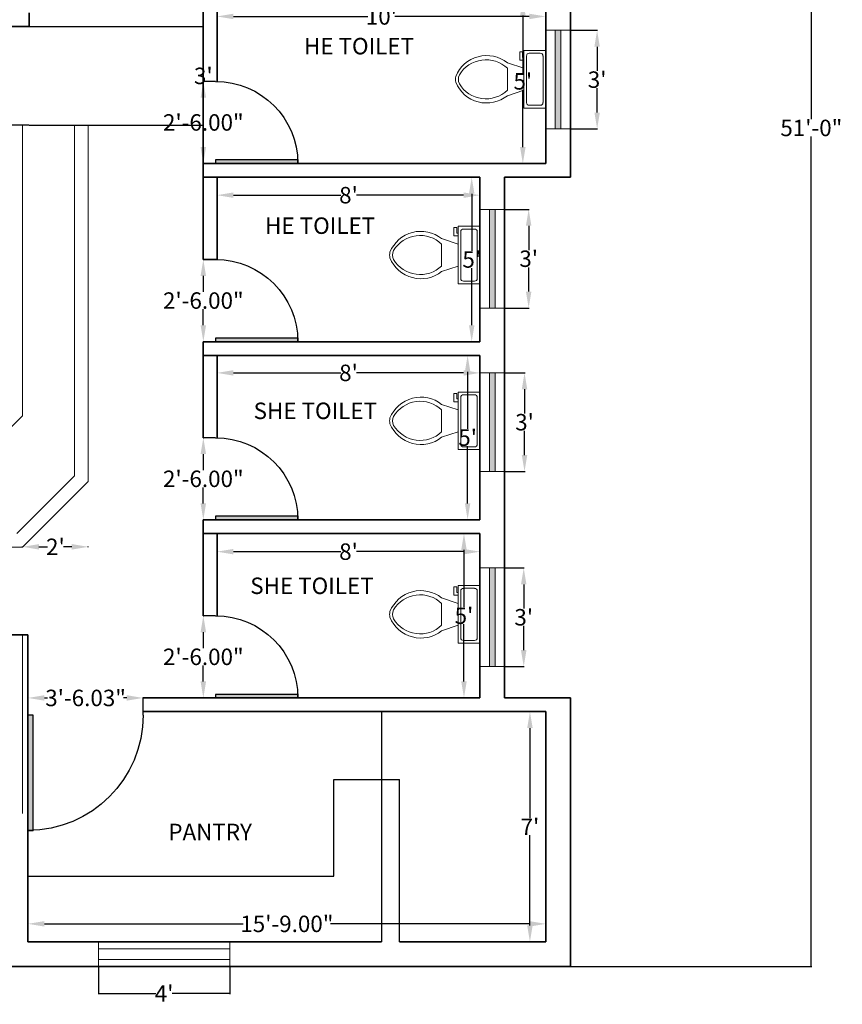
# Model space of a CAD drawing. Units: inches. Extents: x -57 to 1512, y -896 to 149.
# Tile 5 of 6: x 1211 to 1512, y -620 to -261. Entities that reach past the tile are written whole.
import ezdxf

# ---------------------------------------------------------------- set-up
doc = ezdxf.new("R2010")
doc.units = ezdxf.units.IN
doc.header["$MEASUREMENT"] = 0
doc.layers.get('Defpoints').update_dxf_attribs({"color": 9})
for name, color, linetype, lineweight in [('A-ANNO-DIMS', 2, 'Continuous', 18), ('A-AREA-IDEN', 7, 'Continuous', 18), ('A-DOOR', 3, 'Continuous', 25), ('A-DOOR-PATT', 3, 'Continuous', 13), ('A-FLOR-CASE', 8, 'Continuous', 25), ('A-FLOR-FIXT', 9, 'Continuous', 18), ('A-FURN', 8, 'Continuous', 18), ('A-GLAZ', 4, 'Continuous', 18), ('A-GLAZ-PATT', 4, 'Continuous', 13), ('A-WALL', 7, 'Continuous', 35)]:
    doc.layers.add(name, color=color, linetype=linetype, lineweight=lineweight)
doc.styles.get("Standard").update_dxf_attribs({"font": 'arial.ttf'})
doc.dimstyles.get("Standard").update_dxf_attribs({"dimtxt": 6, "dimasz": 0.18, "dimexe": 0.18, "dimexo": 0.0625, "dimgap": 0.09, "dimtad": 0, "dimtih": 1, "dimtoh": 1, "dimzin": 0, "dimdsep": 46, "dimlunit": 3, "dimtxsty": 'Standard', "dimcen": 0.09, "dimadec": 0, "dimazin": 0, "dimtfac": 1, "dimtofl": 0, "dimtmove": 0, "dimatfit": 3, "dimfxl": 1, "dimtolj": 1, "dimtzin": 0, "dimarcsym": 0})

# ---------------------------------------------------------------- blocks, each defined once
blk = doc.blocks.new('*U2')
for p, q in [((0, 0), (0, -6)), ((40, 0), (40, -6))]:
    blk.add_line(p, q)
blk.add_lwpolyline([(0, 0), (0, 40), (1.75, 40), (1.75, 0)], close=True)
blk.add_arc((0, 0), 40, 0, 90)
blk = doc.blocks.new('*D30')
at = {"layer": 'A-ANNO-DIMS', "color": 0, "lineweight": -2, "transparency": 16777216}
for p, q in [((1214.47, -508.36), (1214.47, -508.24)), ((1220.47, -508.42), (1221.6, -508.42)), ((1250.5, -508.42), (1249.37, -508.42)), ((1256.5, -508.36), (1256.5, -508.24))]:
    blk.add_line(p, q, dxfattribs=at)
at = {"layer": 'A-ANNO-DIMS', "color": 0, "transparency": 16777216}
for points in [[(1220.47, -507.42), (1220.47, -509.42), (1214.47, -508.42)], [(1250.5, -507.42), (1250.5, -509.42), (1256.5, -508.42)]]:
    blk.add_solid(points, dxfattribs=at)
at = {"layer": 'Defpoints', "color": 0, "transparency": 16777216}
for p in [(1214.47, -508.42), (1214.47, -508.42), (1256.5, -508.42)]:
    blk.add_point(p, dxfattribs=at)
at = {"layer": 'A-ANNO-DIMS', "color": 0, "transparency": 16777216, "insert": (1235.49, -508.42), "char_height": 6, "attachment_point": 5}
blk.add_mtext('\\A1;3\'-6.03"', dxfattribs=at)
blk = doc.blocks.new('*D31')
at = {"layer": 'A-ANNO-DIMS', "color": 0, "lineweight": -2, "transparency": 16777216}
for p, q in [((1278.53, -478.42), (1278.65, -478.42)), ((1278.47, -484.42), (1278.47, -490.27)), ((1278.47, -502.42), (1278.47, -496.58)), ((1278.53, -508.42), (1278.65, -508.42))]:
    blk.add_line(p, q, dxfattribs=at)
at = {"layer": 'A-ANNO-DIMS', "color": 0, "transparency": 16777216}
for points in [[(1277.47, -484.42), (1279.47, -484.42), (1278.47, -478.42)], [(1277.47, -502.42), (1279.47, -502.42), (1278.47, -508.42)]]:
    blk.add_solid(points, dxfattribs=at)
at = {"layer": 'Defpoints', "color": 0, "transparency": 16777216}
for p in [(1278.47, -478.42), (1278.47, -508.42), (1278.47, -508.42)]:
    blk.add_point(p, dxfattribs=at)
at = {"layer": 'A-ANNO-DIMS', "color": 0, "transparency": 16777216, "insert": (1278.47, -493.42), "char_height": 6, "attachment_point": 5}
blk.add_mtext('\\A1;2\'-6.00"', dxfattribs=at)
blk = doc.blocks.new('*D32')
at = {"layer": 'A-ANNO-DIMS', "color": 0, "lineweight": -2, "transparency": 16777216}
for p, q in [((1278.53, -413.46), (1278.65, -413.46)), ((1278.47, -419.46), (1278.47, -425.31)), ((1278.47, -437.46), (1278.47, -431.61)), ((1278.53, -443.46), (1278.65, -443.46))]:
    blk.add_line(p, q, dxfattribs=at)
at = {"layer": 'A-ANNO-DIMS', "color": 0, "transparency": 16777216}
for points in [[(1277.47, -419.46), (1279.47, -419.46), (1278.47, -413.46)], [(1277.47, -437.46), (1279.47, -437.46), (1278.47, -443.46)]]:
    blk.add_solid(points, dxfattribs=at)
at = {"layer": 'Defpoints', "color": 0, "transparency": 16777216}
for p in [(1278.47, -413.46), (1278.47, -443.46), (1278.47, -443.46)]:
    blk.add_point(p, dxfattribs=at)
at = {"layer": 'A-ANNO-DIMS', "color": 0, "transparency": 16777216, "insert": (1278.47, -428.46), "char_height": 6, "attachment_point": 5}
blk.add_mtext('\\A1;2\'-6.00"', dxfattribs=at)
blk = doc.blocks.new('*D33')
at = {"layer": 'A-ANNO-DIMS', "color": 0, "lineweight": -2, "transparency": 16777216}
for p, q in [((1278.53, -348.42), (1278.65, -348.42)), ((1278.47, -354.42), (1278.47, -360.27)), ((1278.47, -372.42), (1278.47, -366.58)), ((1278.53, -378.42), (1278.65, -378.42))]:
    blk.add_line(p, q, dxfattribs=at)
at = {"layer": 'A-ANNO-DIMS', "color": 0, "transparency": 16777216}
for points in [[(1277.47, -354.42), (1279.47, -354.42), (1278.47, -348.42)], [(1277.47, -372.42), (1279.47, -372.42), (1278.47, -378.42)]]:
    blk.add_solid(points, dxfattribs=at)
at = {"layer": 'Defpoints', "color": 0, "transparency": 16777216}
for p in [(1278.47, -348.42), (1278.47, -378.42), (1278.47, -378.42)]:
    blk.add_point(p, dxfattribs=at)
at = {"layer": 'A-ANNO-DIMS', "color": 0, "transparency": 16777216, "insert": (1278.47, -363.42), "char_height": 6, "attachment_point": 5}
blk.add_mtext('\\A1;2\'-6.00"', dxfattribs=at)
blk = doc.blocks.new('*D34')
at = {"layer": 'A-ANNO-DIMS', "color": 0, "lineweight": -2, "transparency": 16777216}
for p, q in [((1278.53, -283.42), (1278.65, -283.42)), ((1278.47, -289.42), (1278.47, -295.27)), ((1278.47, -307.42), (1278.47, -301.58)), ((1278.53, -313.42), (1278.65, -313.42))]:
    blk.add_line(p, q, dxfattribs=at)
at = {"layer": 'A-ANNO-DIMS', "color": 0, "transparency": 16777216}
for points in [[(1277.47, -289.42), (1279.47, -289.42), (1278.47, -283.42)], [(1277.47, -307.42), (1279.47, -307.42), (1278.47, -313.42)]]:
    blk.add_solid(points, dxfattribs=at)
at = {"layer": 'Defpoints', "color": 0, "transparency": 16777216}
for p in [(1278.47, -283.42), (1278.47, -313.42), (1278.47, -313.42)]:
    blk.add_point(p, dxfattribs=at)
at = {"layer": 'A-ANNO-DIMS', "color": 0, "transparency": 16777216, "insert": (1278.47, -298.42), "char_height": 6, "attachment_point": 5}
blk.add_mtext('\\A1;2\'-6.00"', dxfattribs=at)
blk = doc.blocks.new('*D44')
at = {"layer": 'A-ANNO-DIMS', "color": 0, "lineweight": -2, "transparency": 16777216}
for p, q in [((1240.15, -606.48), (1240.15, -616.46)), ((1288.15, -606.48), (1288.15, -616.46)), ((1240.33, -616.28), (1261.17, -616.28)), ((1287.97, -616.28), (1267.12, -616.28))]:
    blk.add_line(p, q, dxfattribs=at)
at = {"layer": 'A-ANNO-DIMS', "color": 0, "transparency": 16777216}
for points in [[(1240.33, -616.25), (1240.33, -616.31), (1240.15, -616.28)], [(1287.97, -616.25), (1287.97, -616.31), (1288.15, -616.28)]]:
    blk.add_solid(points, dxfattribs=at)
at = {"layer": 'Defpoints', "color": 0, "transparency": 16777216}
for p in [(1240.15, -606.42), (1288.15, -606.42), (1288.15, -616.28)]:
    blk.add_point(p, dxfattribs=at)
at = {"layer": 'A-ANNO-DIMS', "color": 0, "transparency": 16777216, "insert": (1264.15, -616.28), "char_height": 6, "attachment_point": 5}
blk.add_mtext("\\A1;4'", dxfattribs=at)
blk = doc.blocks.new('*D45')
at = {"layer": 'A-ANNO-DIMS', "color": 0, "lineweight": -2, "transparency": 16777216}
for p, q in [((1388.53, -330.14), (1397.42, -330.14)), ((1397.24, -336.14), (1397.24, -344.99)), ((1397.24, -360.14), (1397.24, -351.3)), ((1388.53, -366.14), (1397.42, -366.14))]:
    blk.add_line(p, q, dxfattribs=at)
at = {"layer": 'A-ANNO-DIMS', "color": 0, "transparency": 16777216}
for points in [[(1396.24, -336.14), (1398.24, -336.14), (1397.24, -330.14)], [(1396.24, -360.14), (1398.24, -360.14), (1397.24, -366.14)]]:
    blk.add_solid(points, dxfattribs=at)
at = {"layer": 'Defpoints', "color": 0, "transparency": 16777216}
for p in [(1388.47, -330.14), (1388.47, -366.14), (1397.24, -366.14)]:
    blk.add_point(p, dxfattribs=at)
at = {"layer": 'A-ANNO-DIMS', "color": 0, "transparency": 16777216, "insert": (1397.24, -348.14), "char_height": 6, "attachment_point": 5}
blk.add_mtext("\\A1;3'", dxfattribs=at)
blk = doc.blocks.new('*D46')
at = {"layer": 'A-ANNO-DIMS', "color": 0, "lineweight": -2, "transparency": 16777216}
for p, q in [((1388.53, -389.8), (1395.91, -389.8)), ((1395.73, -395.8), (1395.73, -404.65)), ((1395.73, -419.8), (1395.73, -410.96)), ((1388.53, -425.8), (1395.91, -425.8))]:
    blk.add_line(p, q, dxfattribs=at)
at = {"layer": 'A-ANNO-DIMS', "color": 0, "transparency": 16777216}
for points in [[(1394.73, -395.8), (1396.73, -395.8), (1395.73, -389.8)], [(1394.73, -419.8), (1396.73, -419.8), (1395.73, -425.8)]]:
    blk.add_solid(points, dxfattribs=at)
at = {"layer": 'Defpoints', "color": 0, "transparency": 16777216}
for p in [(1388.47, -389.8), (1388.47, -425.8), (1395.73, -425.8)]:
    blk.add_point(p, dxfattribs=at)
at = {"layer": 'A-ANNO-DIMS', "color": 0, "transparency": 16777216, "insert": (1395.73, -407.8), "char_height": 6, "attachment_point": 5}
blk.add_mtext("\\A1;3'", dxfattribs=at)
blk = doc.blocks.new('*D47')
at = {"layer": 'A-ANNO-DIMS', "color": 0, "lineweight": -2, "transparency": 16777216}
for p, q in [((1388.53, -460.98), (1395.61, -460.98)), ((1395.43, -466.98), (1395.43, -475.83)), ((1395.43, -490.98), (1395.43, -482.14)), ((1388.53, -496.98), (1395.61, -496.98))]:
    blk.add_line(p, q, dxfattribs=at)
at = {"layer": 'A-ANNO-DIMS', "color": 0, "transparency": 16777216}
for points in [[(1394.43, -466.98), (1396.43, -466.98), (1395.43, -460.98)], [(1394.43, -490.98), (1396.43, -490.98), (1395.43, -496.98)]]:
    blk.add_solid(points, dxfattribs=at)
at = {"layer": 'Defpoints', "color": 0, "transparency": 16777216}
for p in [(1388.47, -460.98), (1395.43, -460.98), (1388.47, -496.98)]:
    blk.add_point(p, dxfattribs=at)
at = {"layer": 'A-ANNO-DIMS', "color": 0, "transparency": 16777216, "insert": (1395.43, -478.98), "char_height": 6, "attachment_point": 5}
blk.add_mtext("\\A1;3'", dxfattribs=at)
blk = doc.blocks.new('*D48')
at = {"layer": 'A-ANNO-DIMS', "color": 0, "lineweight": -2, "transparency": 16777216}
for p, q in [((1412.53, -264.79), (1422.41, -264.79)), ((1422.23, -270.79), (1422.23, -279.64)), ((1422.23, -294.79), (1422.23, -285.95)), ((1412.53, -300.79), (1422.41, -300.79))]:
    blk.add_line(p, q, dxfattribs=at)
at = {"layer": 'A-ANNO-DIMS', "color": 0, "transparency": 16777216}
for points in [[(1421.23, -270.79), (1423.23, -270.79), (1422.23, -264.79)], [(1421.23, -294.79), (1423.23, -294.79), (1422.23, -300.79)]]:
    blk.add_solid(points, dxfattribs=at)
at = {"layer": 'Defpoints', "color": 0, "transparency": 16777216}
for p in [(1412.47, -264.79), (1412.47, -300.79), (1422.23, -300.79)]:
    blk.add_point(p, dxfattribs=at)
at = {"layer": 'A-ANNO-DIMS', "color": 0, "transparency": 16777216, "insert": (1422.23, -282.79), "char_height": 6, "attachment_point": 5}
blk.add_mtext("\\A1;3'", dxfattribs=at)
blk = doc.blocks.new('*U24')
for p, q in [((9.5, -6), (9.5, -2)), ((-10, -8.5), (-8, -8.5)), ((-10, -9.5), (-10, -8.5)), ((-7, -9.5), (-10, -9.5)), ((-8, -8.5), (-8, -8)), ((-7, -8), (-7, -9.5)), ((-4, -8), (-6, -14)), ((4, -8), (6, -14)), ((4, -14), (-4, -14))]:
    blk.add_line(p, q)
blk.add_lwpolyline([(10.5, -8), (10.5, 0), (-10.5, 0), (-10.5, -8)], close=True)
for points in [[(-9.5, -2), (-9.5, -6)], [(8.5, -1), (-8.5, -1)], [(-8.5, -7), (8.5, -7)]]:
    blk.add_lwpolyline(points)
for centre, radius, start, end in [((-8.62, -1.88), 0.884, 81.8699, 188.1301), ((8.62, -1.88), 0.884, 351.8699, 98.1301), ((-8.62, -6.12), 0.884, 171.8699, 278.1301), ((8.62, -6.12), 0.884, 261.8699, 8.1301), ((3.52, -21.58), 12.17, 141.4691, 247.9714), ((4.2, -21.82), 11.33, 136.3677, 238.9468), ((-3.52, -21.58), 12.17, 292.0284, 38.5307), ((-4.2, -21.82), 11.33, 301.053, 43.6321), ((0, -27.88), 4, 245.7318, 294.2682), ((0, -29), 4, 254.8605, 285.1395)]:
    blk.add_arc(centre, radius, start, end)
blk = doc.blocks.new('*D57')
at = {"layer": 'A-ANNO-DIMS', "color": 0, "lineweight": -2, "transparency": 16777216}
for p, q in [((1214.95, -263.42), (1278.65, -263.42)), ((1278.47, -263.6), (1278.47, -278.27)), ((1278.47, -299.24), (1278.47, -284.58)), ((1214.95, -299.42), (1278.65, -299.42))]:
    blk.add_line(p, q, dxfattribs=at)
at = {"layer": 'A-ANNO-DIMS', "color": 0, "transparency": 16777216}
for points in [[(1278.44, -263.6), (1278.5, -263.6), (1278.47, -263.42)], [(1278.44, -299.24), (1278.5, -299.24), (1278.47, -299.42)]]:
    blk.add_solid(points, dxfattribs=at)
at = {"layer": 'Defpoints', "color": 0, "transparency": 16777216}
for p in [(1214.89, -263.42), (1214.89, -299.42), (1278.47, -299.42)]:
    blk.add_point(p, dxfattribs=at)
at = {"layer": 'A-ANNO-DIMS', "color": 0, "transparency": 16777216, "insert": (1278.47, -281.42), "char_height": 6, "attachment_point": 5}
blk.add_mtext("\\A1;3'", dxfattribs=at)
blk = doc.blocks.new('*D58')
at = {"layer": 'A-ANNO-DIMS', "color": 0, "lineweight": -2, "transparency": 16777216}
for p, q in [((1214.83, -263.42), (1191.49, -263.42)), ((1191.67, -269.42), (1191.67, -278.27)), ((1191.67, -293.42), (1191.67, -284.58)), ((1214.83, -299.42), (1191.49, -299.42))]:
    blk.add_line(p, q, dxfattribs=at)
at = {"layer": 'A-ANNO-DIMS', "color": 0, "transparency": 16777216}
for points in [[(1190.67, -269.42), (1192.67, -269.42), (1191.67, -263.42)], [(1190.67, -293.42), (1192.67, -293.42), (1191.67, -299.42)]]:
    blk.add_solid(points, dxfattribs=at)
at = {"layer": 'Defpoints', "color": 0, "transparency": 16777216}
for p in [(1214.89, -263.42), (1191.67, -299.42), (1214.89, -299.42)]:
    blk.add_point(p, dxfattribs=at)
at = {"layer": 'A-ANNO-DIMS', "color": 0, "transparency": 16777216, "insert": (1191.67, -281.42), "char_height": 6, "attachment_point": 5}
blk.add_mtext("\\A1;3'", dxfattribs=at)
blk = doc.blocks.new('*D61')
at = {"layer": 'A-ANNO-DIMS', "color": 0, "lineweight": -2, "transparency": 16777216}
for p, q in [((1212.47, -453.36), (1212.47, -453.1)), ((1218.47, -453.28), (1221.57, -453.28)), ((1230.47, -453.28), (1227.37, -453.28)), ((1236.47, -453.36), (1236.47, -453.1))]:
    blk.add_line(p, q, dxfattribs=at)
at = {"layer": 'A-ANNO-DIMS', "color": 0, "transparency": 16777216}
for points in [[(1218.47, -452.28), (1218.47, -454.28), (1212.47, -453.28)], [(1230.47, -452.28), (1230.47, -454.28), (1236.47, -453.28)]]:
    blk.add_solid(points, dxfattribs=at)
at = {"layer": 'Defpoints', "color": 0, "transparency": 16777216}
for p in [(1212.47, -453.42), (1236.47, -453.28), (1236.47, -453.42)]:
    blk.add_point(p, dxfattribs=at)
at = {"layer": 'A-ANNO-DIMS', "color": 0, "transparency": 16777216, "insert": (1224.47, -453.28), "char_height": 6, "attachment_point": 5}
blk.add_mtext("\\A1;2'", dxfattribs=at)
blk = doc.blocks.new('*D62')
at = {"layer": 'A-ANNO-DIMS', "color": 0, "lineweight": -2, "transparency": 16777216}
for p, q in [((1283.47, -253.48), (1283.47, -259.92)), ((1403.47, -253.48), (1403.47, -259.92)), ((1289.47, -259.74), (1338.57, -259.74)), ((1397.47, -259.74), (1348.37, -259.74))]:
    blk.add_line(p, q, dxfattribs=at)
at = {"layer": 'A-ANNO-DIMS', "color": 0, "transparency": 16777216}
for points in [[(1289.47, -258.74), (1289.47, -260.74), (1283.47, -259.74)], [(1397.47, -258.74), (1397.47, -260.74), (1403.47, -259.74)]]:
    blk.add_solid(points, dxfattribs=at)
at = {"layer": 'Defpoints', "color": 0, "transparency": 16777216}
for p in [(1283.47, -253.42), (1403.47, -253.42), (1403.47, -259.74)]:
    blk.add_point(p, dxfattribs=at)
at = {"layer": 'A-ANNO-DIMS', "color": 0, "transparency": 16777216, "insert": (1343.47, -259.74), "char_height": 6, "attachment_point": 5}
blk.add_mtext("\\A1;10'", dxfattribs=at)
blk = doc.blocks.new('*D63')
at = {"layer": 'A-ANNO-DIMS', "color": 0, "lineweight": -2, "transparency": 16777216}
for p, q in [((1403.41, -253.42), (1394.93, -253.42)), ((1395.11, -259.42), (1395.11, -280.28)), ((1395.11, -307.42), (1395.11, -286.56)), ((1403.41, -313.42), (1394.93, -313.42))]:
    blk.add_line(p, q, dxfattribs=at)
at = {"layer": 'A-ANNO-DIMS', "color": 0, "transparency": 16777216}
for points in [[(1394.11, -259.42), (1396.11, -259.42), (1395.11, -253.42)], [(1394.11, -307.42), (1396.11, -307.42), (1395.11, -313.42)]]:
    blk.add_solid(points, dxfattribs=at)
at = {"layer": 'Defpoints', "color": 0, "transparency": 16777216}
for p in [(1395.11, -253.42), (1403.47, -253.42), (1403.47, -313.42)]:
    blk.add_point(p, dxfattribs=at)
at = {"layer": 'A-ANNO-DIMS', "color": 0, "transparency": 16777216, "insert": (1395.11, -283.42), "char_height": 6, "attachment_point": 5}
blk.add_mtext("\\A1;5'", dxfattribs=at)
blk = doc.blocks.new('*D64')
at = {"layer": 'A-ANNO-DIMS', "color": 0, "lineweight": -2, "transparency": 16777216}
for p, q in [((1283.47, -324.89), (1283.47, -324.77)), ((1289.47, -324.95), (1328.62, -324.95)), ((1373.47, -324.95), (1334.33, -324.95)), ((1379.47, -324.89), (1379.47, -324.77))]:
    blk.add_line(p, q, dxfattribs=at)
at = {"layer": 'A-ANNO-DIMS', "color": 0, "transparency": 16777216}
for points in [[(1289.47, -323.95), (1289.47, -325.95), (1283.47, -324.95)], [(1373.47, -323.95), (1373.47, -325.95), (1379.47, -324.95)]]:
    blk.add_solid(points, dxfattribs=at)
at = {"layer": 'Defpoints', "color": 0, "transparency": 16777216}
for p in [(1283.47, -324.95), (1379.47, -324.95), (1379.47, -324.95)]:
    blk.add_point(p, dxfattribs=at)
at = {"layer": 'A-ANNO-DIMS', "color": 0, "transparency": 16777216, "insert": (1331.47, -324.95), "char_height": 6, "attachment_point": 5}
blk.add_mtext("\\A1;8'", dxfattribs=at)
blk = doc.blocks.new('*D65')
at = {"layer": 'A-ANNO-DIMS', "color": 0, "lineweight": -2, "transparency": 16777216}
for p, q in [((1379.41, -318.42), (1376.27, -318.42)), ((1376.45, -324.42), (1376.45, -345.28)), ((1376.45, -372.42), (1376.45, -351.56)), ((1379.41, -378.42), (1376.27, -378.42))]:
    blk.add_line(p, q, dxfattribs=at)
at = {"layer": 'A-ANNO-DIMS', "color": 0, "transparency": 16777216}
for points in [[(1375.45, -324.42), (1377.45, -324.42), (1376.45, -318.42)], [(1375.45, -372.42), (1377.45, -372.42), (1376.45, -378.42)]]:
    blk.add_solid(points, dxfattribs=at)
at = {"layer": 'Defpoints', "color": 0, "transparency": 16777216}
for p in [(1379.47, -318.42), (1376.45, -378.42), (1379.47, -378.42)]:
    blk.add_point(p, dxfattribs=at)
at = {"layer": 'A-ANNO-DIMS', "color": 0, "transparency": 16777216, "insert": (1376.45, -348.42), "char_height": 6, "attachment_point": 5}
blk.add_mtext("\\A1;5'", dxfattribs=at)
blk = doc.blocks.new('*D66')
at = {"layer": 'A-ANNO-DIMS', "color": 0, "lineweight": -2, "transparency": 16777216}
for p, q in [((1379.41, -383.42), (1374.77, -383.42)), ((1374.95, -389.42), (1374.95, -410.28)), ((1374.95, -437.42), (1374.95, -416.56)), ((1379.41, -443.42), (1374.77, -443.42))]:
    blk.add_line(p, q, dxfattribs=at)
at = {"layer": 'A-ANNO-DIMS', "color": 0, "transparency": 16777216}
for points in [[(1373.95, -389.42), (1375.95, -389.42), (1374.95, -383.42)], [(1373.95, -437.42), (1375.95, -437.42), (1374.95, -443.42)]]:
    blk.add_solid(points, dxfattribs=at)
at = {"layer": 'Defpoints', "color": 0, "transparency": 16777216}
for p in [(1379.47, -383.42), (1374.95, -443.42), (1379.47, -443.42)]:
    blk.add_point(p, dxfattribs=at)
at = {"layer": 'A-ANNO-DIMS', "color": 0, "transparency": 16777216, "insert": (1374.95, -413.42), "char_height": 6, "attachment_point": 5}
blk.add_mtext("\\A1;5'", dxfattribs=at)
blk = doc.blocks.new('*D67')
at = {"layer": 'A-ANNO-DIMS', "color": 0, "lineweight": -2, "transparency": 16777216}
for p, q in [((1379.41, -448.42), (1373.44, -448.42)), ((1373.62, -454.42), (1373.62, -475.28)), ((1373.62, -502.42), (1373.62, -481.56)), ((1379.41, -508.42), (1373.44, -508.42))]:
    blk.add_line(p, q, dxfattribs=at)
at = {"layer": 'A-ANNO-DIMS', "color": 0, "transparency": 16777216}
for points in [[(1372.62, -454.42), (1374.62, -454.42), (1373.62, -448.42)], [(1372.62, -502.42), (1374.62, -502.42), (1373.62, -508.42)]]:
    blk.add_solid(points, dxfattribs=at)
at = {"layer": 'Defpoints', "color": 0, "transparency": 16777216}
for p in [(1379.47, -448.42), (1373.62, -508.42), (1379.47, -508.42)]:
    blk.add_point(p, dxfattribs=at)
at = {"layer": 'A-ANNO-DIMS', "color": 0, "transparency": 16777216, "insert": (1373.62, -478.42), "char_height": 6, "attachment_point": 5}
blk.add_mtext("\\A1;5'", dxfattribs=at)
blk = doc.blocks.new('*D68')
at = {"layer": 'A-ANNO-DIMS', "color": 0, "lineweight": -2, "transparency": 16777216}
for p, q in [((1283.47, -383.48), (1283.47, -389.98)), ((1379.47, -383.66), (1379.47, -389.98)), ((1289.47, -389.8), (1328.62, -389.8)), ((1373.47, -389.8), (1334.33, -389.8))]:
    blk.add_line(p, q, dxfattribs=at)
at = {"layer": 'A-ANNO-DIMS', "color": 0, "transparency": 16777216}
for points in [[(1289.47, -388.8), (1289.47, -390.8), (1283.47, -389.8)], [(1373.47, -388.8), (1373.47, -390.8), (1379.47, -389.8)]]:
    blk.add_solid(points, dxfattribs=at)
at = {"layer": 'Defpoints', "color": 0, "transparency": 16777216}
for p in [(1283.47, -383.42), (1379.47, -383.6), (1379.47, -389.8)]:
    blk.add_point(p, dxfattribs=at)
at = {"layer": 'A-ANNO-DIMS', "color": 0, "transparency": 16777216, "insert": (1331.47, -389.8), "char_height": 6, "attachment_point": 5}
blk.add_mtext("\\A1;8'", dxfattribs=at)
blk = doc.blocks.new('*D69')
at = {"layer": 'A-ANNO-DIMS', "color": 0, "lineweight": -2, "transparency": 16777216}
for p, q in [((1283.47, -448.48), (1283.47, -455.22)), ((1379.47, -448.48), (1379.47, -455.22)), ((1289.47, -455.04), (1328.62, -455.04)), ((1373.47, -455.04), (1334.33, -455.04))]:
    blk.add_line(p, q, dxfattribs=at)
at = {"layer": 'A-ANNO-DIMS', "color": 0, "transparency": 16777216}
for points in [[(1289.47, -454.04), (1289.47, -456.04), (1283.47, -455.04)], [(1373.47, -454.04), (1373.47, -456.04), (1379.47, -455.04)]]:
    blk.add_solid(points, dxfattribs=at)
at = {"layer": 'Defpoints', "color": 0, "transparency": 16777216}
for p in [(1283.47, -448.42), (1379.47, -448.42), (1379.47, -455.04)]:
    blk.add_point(p, dxfattribs=at)
at = {"layer": 'A-ANNO-DIMS', "color": 0, "transparency": 16777216, "insert": (1331.47, -455.04), "char_height": 6, "attachment_point": 5}
blk.add_mtext("\\A1;8'", dxfattribs=at)
blk = doc.blocks.new('*D70')
at = {"layer": 'A-ANNO-DIMS', "color": 0, "lineweight": -2, "transparency": 16777216}
for p, q in [((1214.47, -597.36), (1214.47, -590.68)), ((1220.47, -590.86), (1293.03, -590.86)), ((1397.47, -590.86), (1324.91, -590.86)), ((1403.47, -597.36), (1403.47, -590.68))]:
    blk.add_line(p, q, dxfattribs=at)
at = {"layer": 'A-ANNO-DIMS', "color": 0, "transparency": 16777216}
for points in [[(1220.47, -589.86), (1220.47, -591.86), (1214.47, -590.86)], [(1397.47, -589.86), (1397.47, -591.86), (1403.47, -590.86)]]:
    blk.add_solid(points, dxfattribs=at)
at = {"layer": 'Defpoints', "color": 0, "transparency": 16777216}
for p in [(1403.47, -590.86), (1214.47, -597.42), (1403.47, -597.42)]:
    blk.add_point(p, dxfattribs=at)
at = {"layer": 'A-ANNO-DIMS', "color": 0, "transparency": 16777216, "insert": (1308.97, -590.86), "char_height": 6, "attachment_point": 5}
blk.add_mtext('\\A1;15\'-9.00"', dxfattribs=at)
blk = doc.blocks.new('*D71')
at = {"layer": 'A-ANNO-DIMS', "color": 0, "lineweight": -2, "transparency": 16777216}
for p, q in [((1403.41, -513.42), (1397.52, -513.42)), ((1397.7, -519.42), (1397.7, -552.33)), ((1397.7, -591.42), (1397.7, -558.51)), ((1403.41, -597.42), (1397.52, -597.42))]:
    blk.add_line(p, q, dxfattribs=at)
at = {"layer": 'A-ANNO-DIMS', "color": 0, "transparency": 16777216}
for points in [[(1396.7, -519.42), (1398.7, -519.42), (1397.7, -513.42)], [(1396.7, -591.42), (1398.7, -591.42), (1397.7, -597.42)]]:
    blk.add_solid(points, dxfattribs=at)
at = {"layer": 'Defpoints', "color": 0, "transparency": 16777216}
for p in [(1397.7, -513.42), (1403.47, -513.42), (1403.47, -597.42)]:
    blk.add_point(p, dxfattribs=at)
at = {"layer": 'A-ANNO-DIMS', "color": 0, "transparency": 16777216, "insert": (1397.7, -555.42), "char_height": 6, "attachment_point": 5}
blk.add_mtext("\\A1;7'", dxfattribs=at)
blk = doc.blocks.new('*D105')
at = {"layer": 'A-ANNO-DIMS', "color": 0, "lineweight": -2, "transparency": 16777216}
for p, q in [((1412.53, 5.58), (1500.6, 5.58)), ((1500.42, 5.4), (1500.42, -297.27)), ((1500.42, -606.24), (1500.42, -303.57)), ((1412.53, -606.42), (1500.6, -606.42))]:
    blk.add_line(p, q, dxfattribs=at)
at = {"layer": 'A-ANNO-DIMS', "color": 0, "transparency": 16777216}
for points in [[(1500.39, 5.4), (1500.45, 5.4), (1500.42, 5.58)], [(1500.39, -606.24), (1500.45, -606.24), (1500.42, -606.42)]]:
    blk.add_solid(points, dxfattribs=at)
at = {"layer": 'Defpoints', "color": 0, "transparency": 16777216}
for p in [(1412.47, 5.58), (1500.42, 5.58), (1412.47, -606.42)]:
    blk.add_point(p, dxfattribs=at)
at = {"layer": 'A-ANNO-DIMS', "color": 0, "transparency": 16777216, "insert": (1500.42, -300.42), "char_height": 6, "attachment_point": 5}
blk.add_mtext('\\A1;51\'-0"', dxfattribs=at)

msp = doc.modelspace()

# ---------------------------------------------------------------- hatches: boundary and pattern name
at = {"layer": 'A-DOOR-PATT'}
h = msp.add_hatch(color=256, dxfattribs=at)
h.dxf.hatch_style = 1
h.paths.add_polyline_path([(1084.811, -453.421), (1053.741, -453.421, 0.0109414), (1053.771, -454.781), (1084.811, -454.781)])
h.paths.add_polyline_path([(1091.31, -491.725), (1089.471, -491.725), (1089.471, -533.753), (1091.31, -533.753)])
h.paths.add_polyline_path([(1216.31, -514.725), (1214.471, -514.725), (1214.471, -556.753, 0.0109414), (1216.31, -556.713)])
h.paths.add_polyline_path([(1312.941, -507.109), (1282.971, -507.109), (1282.971, -508.421), (1312.969, -508.421, 0.0109414)])
h.paths.add_polyline_path([(1312.941, -442.147), (1282.971, -442.147), (1282.971, -443.421), (1312.969, -443.421, 0.0106229)])
h.paths.add_polyline_path([(1302.763, -246.583), (1260.775, -246.583), (1260.775, -248.421), (1302.803, -248.421, 0.0109414)])
h.paths.add_polyline_path([(1312.941, -312.109), (1282.971, -312.109), (1282.971, -313.421), (1312.969, -313.421, 0.0109414)])
h.paths.add_polyline_path([(1312.941, -377.109), (1282.971, -377.109), (1282.971, -378.421), (1312.969, -378.421, 0.0109414)])
h.paths.add_polyline_path([(1061.471, -387.473), (1060.289, -387.473), (1060.289, -414.461, 0.0109414), (1061.471, -414.487)])
h.paths.add_polyline_path([(1060.167, -263.421), (1018.139, -263.421, 0.0109414), (1018.179, -265.26), (1060.167, -265.26)])
h.paths.add_polyline_path([(1326.803, -121.583), (1284.775, -121.583), (1284.775, -123.421), (1326.803, -123.421)])
h.paths.add_polyline_path([(980.763, -121.583), (938.775, -121.583), (938.775, -123.421), (980.803, -123.421, 0.0109414)])
h.paths.add_polyline_path([(1177.375, -188.23), (1115.807, -188.23), (1115.807, -219.221), (1177.375, -219.221)])
at = {"layer": 'A-GLAZ-PATT'}
h = msp.add_hatch(color=256, dxfattribs=at)
h.dxf.hatch_style = 1
h.paths.add_polyline_path([(1408.971, -264.791), (1406.971, -264.791), (1406.971, -300.791), (1408.971, -300.791)])
h.paths.add_polyline_path([(1384.971, -330.143), (1382.971, -330.143), (1382.971, -366.143), (1384.971, -366.143)])
h.paths.add_polyline_path([(1384.971, -460.981), (1382.971, -460.981), (1382.971, -496.981), (1384.971, -496.981)])
h.paths.add_polyline_path([(1384.971, -389.802), (1382.971, -389.802), (1382.971, -425.802), (1384.971, -425.802)])
h.paths.add_polyline_path([(937.971, -469.144), (935.971, -469.144), (935.971, -565.144), (937.971, -565.144)])
h.paths.add_polyline_path([(937.971, -399.584), (935.971, -399.584), (935.971, -435.584), (937.971, -435.584)])

# ---------------------------------------------------------------- linework, layer by layer
at = {"layer": 'A-FLOR-CASE'}
for p, q in [((1343.471, -513.421), (1343.471, -597.421)), ((1326.062, -573.421), (1326.062, -538.172)), ((1326.062, -538.172), (1350.062, -538.172)), ((1350.062, -597.421), (1350.062, -538.172)), ((1214.471, -573.421), (1326.062, -573.421))]:
    msp.add_line(p, q, dxfattribs=at)
at = {"layer": 'A-FURN'}
for p, q in [((1038.48, -299.421), (1278.471, -299.421)), ((1212.471, -405.421), (1212.471, -299.421)), ((1231.471, -299.421), (1231.471, -427.35)), ((1236.471, -299.421), (1236.471, -429.421)), ((1188.471, -429.421), (1212.471, -405.421)), ((1210.4, -448.421), (1231.471, -427.35)), ((1212.471, -453.421), (1236.471, -429.421)), ((1132.471, -453.421), (1212.471, -453.421)), ((1212.471, -485.421), (1212.471, -550.535))]:
    msp.add_line(p, q, dxfattribs=at)
at = {"layer": 'A-GLAZ'}
for p, q in [((1403.471, -264.791), (1412.471, -264.791)), ((1406.971, -264.791), (1406.971, -300.791)), ((1408.971, -264.791), (1408.971, -300.791)), ((1403.471, -300.791), (1412.471, -300.791)), ((1379.471, -330.143), (1388.471, -330.143)), ((1382.971, -330.143), (1382.971, -366.143)), ((1384.971, -330.143), (1384.971, -366.143)), ((1379.471, -366.143), (1388.471, -366.143)), ((1379.471, -389.802), (1388.471, -389.802)), ((1382.971, -389.802), (1382.971, -425.802)), ((1384.971, -389.802), (1384.971, -425.802)), ((1379.471, -425.802), (1388.471, -425.802)), ((1379.471, -460.981), (1388.471, -460.981)), ((1382.971, -460.981), (1382.971, -496.981)), ((1384.971, -460.981), (1384.971, -496.981)), ((1379.471, -496.981), (1388.471, -496.981)), ((1240.146, -597.421), (1240.146, -606.421)), ((1240.146, -599.921), (1288.146, -599.921)), ((1288.146, -597.421), (1288.146, -606.421)), ((1240.146, -603.921), (1288.146, -603.921))]:
    msp.add_line(p, q, dxfattribs=at)
at = {"layer": 'A-WALL'}
for p, q in [((1412.471, 5.579), (1412.471, -318.421)), ((1278.471, -253.421), (1278.471, -348.423)), ((1283.471, -253.421), (1283.471, -283.607)), ((1403.471, -253.421), (1403.471, -313.421)), ((1214.89, -258.421), (1214.89, -263.421)), ((941.471, -263.421), (1214.89, -263.421)), ((1278.471, -313.421), (1403.471, -313.421)), ((1278.471, -318.421), (1379.471, -318.421)), ((1283.471, -318.421), (1283.471, -348.427)), ((1379.471, -318.421), (1379.471, -378.421)), ((1388.471, -318.421), (1388.471, -508.421)), ((1388.471, -318.421), (1412.471, -318.421)), ((1278.475, -348.401), (1283.471, -348.401)), ((1379.471, -348.401), (1379.475, -348.401)), ((1278.471, -378.421), (1379.471, -378.421)), ((1278.471, -378.421), (1278.471, -383.421)), ((1278.471, -383.421), (1379.471, -383.421)), ((1278.471, -383.421), (1278.471, -413.461)), ((1283.471, -383.421), (1283.471, -413.465)), ((1379.471, -383.421), (1379.471, -443.421)), ((1278.471, -443.421), (1379.471, -443.421)), ((1278.471, -443.421), (1278.471, -448.421)), ((1278.471, -448.421), (1379.471, -448.421)), ((1278.471, -448.421), (1278.471, -478.423)), ((1283.471, -448.421), (1283.471, -478.427)), ((1379.471, -448.421), (1379.471, -508.421)), ((1131.471, -485.421), (1214.471, -485.421)), ((1214.471, -485.421), (1214.471, -597.421)), ((1256.499, -508.421), (1379.471, -508.421)), ((1388.471, -508.421), (1412.471, -508.421)), ((1412.471, -508.421), (1412.471, -606.421)), ((1256.499, -513.421), (1403.471, -513.421)), ((1403.471, -513.421), (1403.471, -597.421)), ((1214.471, -597.421), (1343.471, -597.421)), ((1350.062, -597.421), (1403.471, -597.421)), ((932.471, -606.421), (1412.471, -606.421))]:
    msp.add_line(p, q, dxfattribs=at)

# ---------------------------------------------------------------- block references
at = {"layer": 'A-DOOR'}
for p, xscale, yscale, zscale, rotation in [((1282.971, -313.421), -0.7499590753743955, 0.7499590753743955, 0.7499590753743955, 270), ((1282.971, -378.421), -0.7499590753743955, 0.7499590753743955, 0.7499590753743955, 270), ((1282.971, -443.459), -0.7499590753743955, 0.7499590753743955, 0.7499590753743955, 270), ((1282.971, -508.421), -0.7499590753743955, 0.7499590753743955, 0.7499590753743955, 270), ((1214.471, -514.725), -1.050697738247698, 1.050697738247698, 1.050697738247698, 180)]:
    msp.add_blockref('*U2', p, dxfattribs=dict(at, xscale=xscale, yscale=yscale, zscale=zscale, rotation=rotation))
at = {"layer": 'A-FLOR-FIXT', "rotation": 270}
for p in [(1403.471, -282.67), (1379.471, -346.804), (1379.471, -407.308), (1379.471, -477.921)]:
    msp.add_blockref('*U24', p, dxfattribs=at)

# ---------------------------------------------------------------- texts
at = {"layer": 'A-AREA-IDEN', "char_height": 6, "attachment_point": 1}
for s, insert in [('HE TOILET', (1315.209, -267.571)), ('HE TOILET', (1301.039, -333.084)), ('SHE TOILET', (1296.832, -400.65)), ('SHE TOILET', (1295.595, -464.5)), ('PANTRY', (1265.709, -554.323))]:
    msp.add_mtext_dynamic_manual_height_columns(s, width=160.11736, gutter_width=1, heights=[0], dxfattribs=dict(at, insert=insert))

# ---------------------------------------------------------------- dimensions: what is measured, and where the dimension line sits
at = {"layer": 'A-ANNO-DIMS'}
for base, p1, p2, override, picture, middle in [((1500.421, 5.579), (1412.471, -606.421), (1412.471, 5.579), {"dimdec": 1, "dimlfac": 1, "dimrnd": 0, "dimzin": 1, "dimdsep": 46, "dimlunit": 4, "dimfrac": 2}, '*D105', (1500.421, -300.421)), ((1395.11, -253.421), (1403.471, -313.421), (1403.471, -253.421), {"dimasz": 6, "dimclrd": 0, "dimclre": 0, "dimclrt": 0}, '*D63', (1395.11, -283.421)), ((1191.669, -299.421), (1214.89, -263.421), (1214.89, -299.421), {"dimasz": 6, "dimclrd": 0, "dimclre": 0, "dimclrt": 0}, '*D58', (1191.669, -281.421)), ((1278.471, -299.421), (1214.89, -263.421), (1214.89, -299.421), {"dimclrd": 0, "dimclre": 0, "dimclrt": 0}, '*D57', (1278.471, -281.421)), ((1422.231, -300.791), (1412.471, -264.791), (1412.471, -300.791), {"dimasz": 6, "dimclrd": 0, "dimclre": 0, "dimclrt": 0}, '*D48', (1422.231, -282.791)), ((1278.471, -313.421), (1278.471, -283.423), (1278.471, -313.421), {"dimasz": 6, "dimclrd": 0, "dimclre": 0, "dimclrt": 0}, '*D34', (1278.471, -298.422)), ((1376.455, -378.421), (1379.471, -318.421), (1379.471, -378.421), {"dimasz": 6, "dimclrd": 0, "dimclre": 0, "dimclrt": 0}, '*D65', (1376.455, -348.421)), ((1397.241, -366.143), (1388.471, -330.143), (1388.471, -366.143), {"dimasz": 6, "dimclrd": 0, "dimclre": 0, "dimclrt": 0}, '*D45', (1397.241, -348.143)), ((1278.471, -378.421), (1278.471, -348.423), (1278.471, -378.421), {"dimasz": 6, "dimclrd": 0, "dimclre": 0, "dimclrt": 0}, '*D33', (1278.471, -363.422)), ((1374.952, -443.421), (1379.471, -383.421), (1379.471, -443.421), {"dimasz": 6, "dimclrd": 0, "dimclre": 0, "dimclrt": 0}, '*D66', (1374.952, -413.421)), ((1395.733, -425.802), (1388.471, -389.802), (1388.471, -425.802), {"dimasz": 6, "dimclrd": 0, "dimclre": 0, "dimclrt": 0}, '*D46', (1395.733, -407.802)), ((1278.471, -443.459), (1278.471, -413.461), (1278.471, -443.459), {"dimasz": 6, "dimclrd": 0, "dimclre": 0, "dimclrt": 0}, '*D32', (1278.471, -428.46)), ((1373.619, -508.421), (1379.471, -448.421), (1379.471, -508.421), {"dimasz": 6, "dimclrd": 0, "dimclre": 0, "dimclrt": 0}, '*D67', (1373.619, -478.421)), ((1395.432, -460.981), (1388.471, -496.981), (1388.471, -460.981), {"dimasz": 6, "dimclrd": 0, "dimclre": 0, "dimclrt": 0}, '*D47', (1395.432, -478.981)), ((1278.471, -508.421), (1278.471, -478.423), (1278.471, -508.421), {"dimasz": 6, "dimclrd": 0, "dimclre": 0, "dimclrt": 0}, '*D31', (1278.471, -493.422)), ((1397.695, -513.421), (1403.471, -597.421), (1403.471, -513.421), {"dimasz": 6, "dimclrd": 0, "dimclre": 0, "dimclrt": 0}, '*D71', (1397.695, -555.421))]:
    dim = msp.add_linear_dim(base=base, p1=p1, p2=p2, angle=90, dimstyle='Standard', override=override, dxfattribs=at)
    dim.commit()
    dim.dimension.update_dxf_attribs({"geometry": picture, "text_midpoint": middle})
for base, p1, p2, override, picture, middle in [((1403.471, -259.741), (1283.471, -253.421), (1403.471, -253.421), {"dimasz": 6, "dimclrd": 0, "dimclre": 0, "dimclrt": 0}, '*D62', (1343.471, -259.741)), ((1379.471, -324.953), (1283.471, -324.953), (1379.471, -324.953), {"dimasz": 6, "dimclrd": 0, "dimclre": 0, "dimclrt": 0}, '*D64', (1331.471, -324.953)), ((1379.471, -389.802), (1283.471, -383.421), (1379.471, -383.601), {"dimasz": 6, "dimclrd": 0, "dimclre": 0, "dimclrt": 0}, '*D68', (1331.471, -389.802)), ((1379.471, -455.037), (1283.471, -448.421), (1379.471, -448.421), {"dimasz": 6, "dimclrd": 0, "dimclre": 0, "dimclrt": 0}, '*D69', (1331.471, -455.037)), ((1236.471, -453.281), (1212.471, -453.421), (1236.471, -453.421), {"dimasz": 6, "dimclrd": 0, "dimclre": 0, "dimclrt": 0}, '*D61', (1224.471, -453.281)), ((1214.471, -508.421), (1256.499, -508.421), (1214.471, -508.421), {"dimasz": 6, "dimclrd": 0, "dimclre": 0, "dimclrt": 0}, '*D30', (1235.485, -508.421)), ((1403.471, -590.863), (1214.471, -597.421), (1403.471, -597.421), {"dimasz": 6, "dimclrd": 0, "dimclre": 0, "dimclrt": 0}, '*D70', (1308.971, -590.863)), ((1288.146, -616.279), (1240.146, -606.421), (1288.146, -606.421), {"dimclrd": 0, "dimclre": 0, "dimclrt": 0}, '*D44', (1264.146, -616.279))]:
    dim = msp.add_linear_dim(base=base, p1=p1, p2=p2, dimstyle='Standard', override=override, dxfattribs=at)
    dim.commit()
    dim.dimension.update_dxf_attribs({"geometry": picture, "text_midpoint": middle})

doc.saveas('drawing.dxf')
